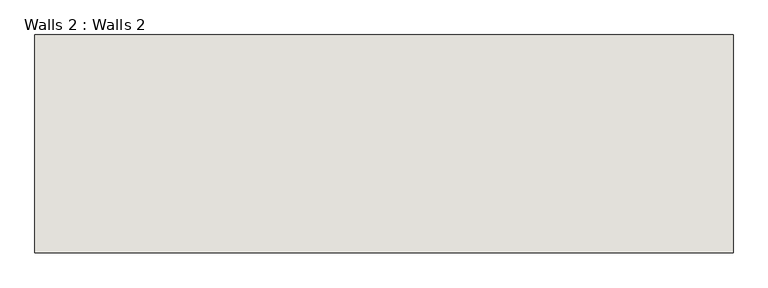
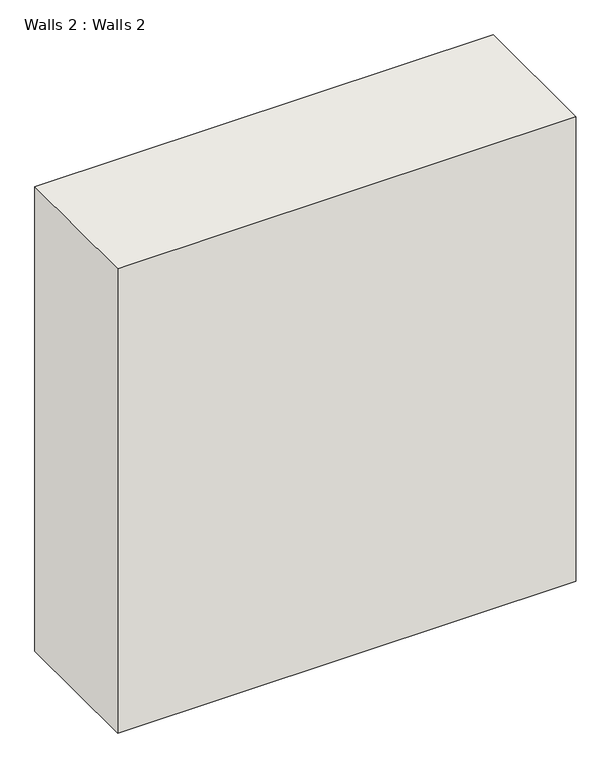
"""IFC4 building model written with IfcOpenShell, lengths in millimetres: wall geometry, Walls 2 : Walls 2."""

from ifc_helpers import new_model, si_unit, frame, origin, place, context, project, spatial, polyline, outline, extrude, source, transform, mapped, element, save


def walls_2_walls_2_a00b9660(model_context):
    return source(origin(), model_context, "Body", "SweptSolid", [
        extrude(outline(polyline([(-2121.6061302, -3147.2991687), (-5213.7749149, -3147.2991687), (-5213.7749149, -2181.7451257), (-2121.6061302, -2181.7451257), (-2121.6061302, -3147.2991687)])), frame((0.0, 0.0, 7620.0), z_axis=(0.0, 0.0, 1.0), x_axis=(1.0, 0.0, 0.0)), (0.0, 0.0, 1.0), 3311.9442033),
    ])


if __name__ == "__main__":
    model = new_model("IFC4")
    model_context = context("Model", 3, world=origin())
    ifc_project = project(units=[si_unit("LENGTHUNIT", "METRE", prefix="MILLI")], contexts=[model_context])
    site = spatial("IfcSite", under=ifc_project)
    building = spatial("IfcBuilding", under=site)
    placement = place(None, origin())
    walls_2_walls_2_shape = walls_2_walls_2_a00b9660(model_context)
    element("IfcWall", 1, ObjectType="Walls 2 : Walls 2", at=placement, inside=building, context=model_context, shape_type="MappedRepresentation", body=[
        mapped(walls_2_walls_2_shape, transform((0.0, 0.0, 0.0), x_axis=(1.0, 0.0, 0.0), y_axis=(0.0, 1.0, 0.0), z_axis=(0.0, 0.0, 1.0))),
    ])
    save(model, "model.ifc")

# Revit data of these elements
# Element 1 (IfcWall, "Walls 2 : Walls 2")
#   Materials on its faces: "Default Wall"
# Materials
#   "Default Wall": colour RGB 128 128 128, transparency 0
